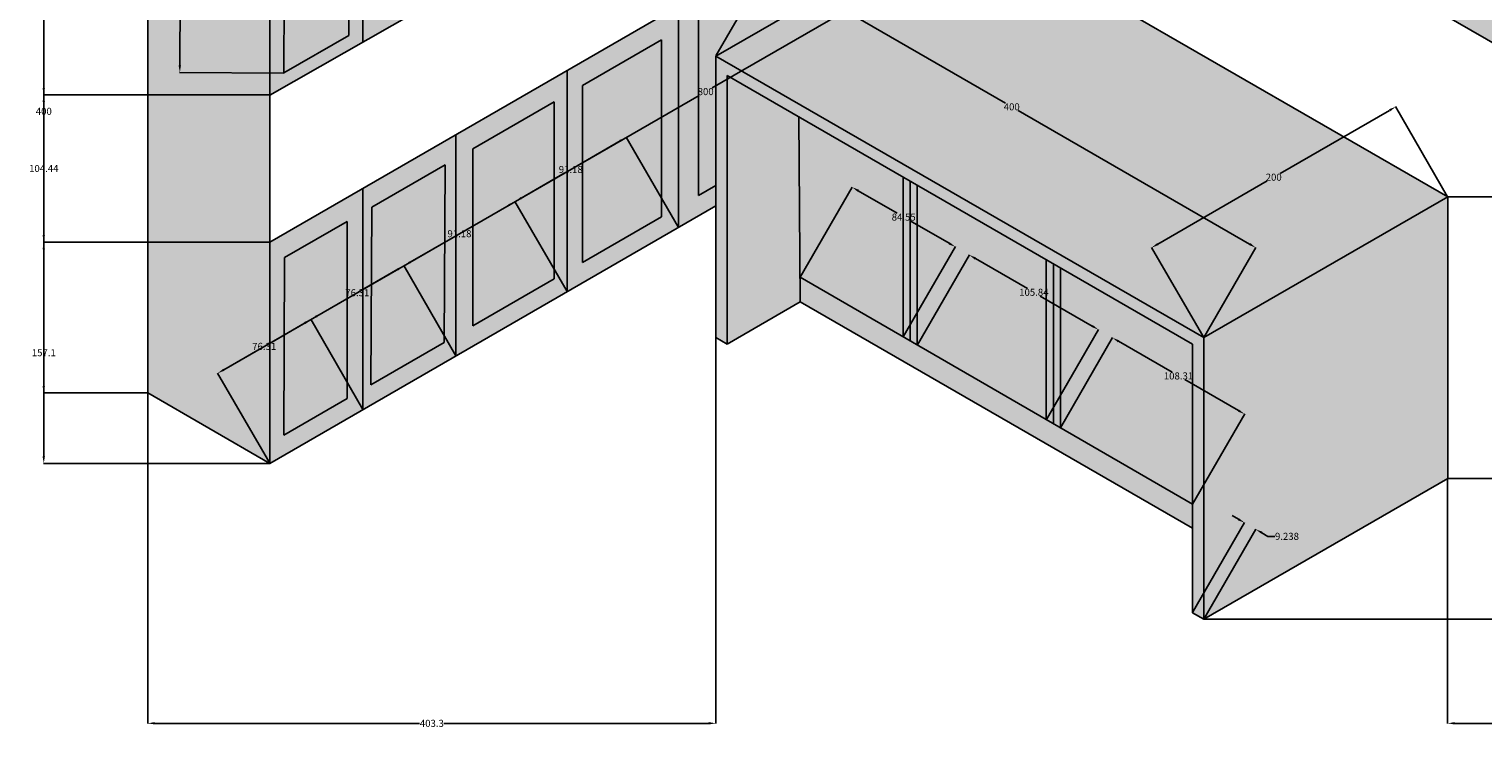
# Model space of a CAD drawing. Units: centimetres. Extents: x -744 to 1642, y 210 to 1375.
# Tile 1 of 8: x -744 to 288, y 210 to 707. Entities that reach past the tile are written whole.
import ezdxf

# ---------------------------------------------------------------- set-up
doc = ezdxf.new("R2010")
doc.units = ezdxf.units.CM
doc.header["$MEASUREMENT"] = 0
for name, color, linetype, lineweight in [('A-ANNO-DIMS', 2, 'Continuous', 18), ('A-EQPM-PATT', 9, 'Continuous', 13), ('A-FURN', 7, 'Continuous', 25), ('A-FURN-PATT', 30, 'Continuous', 13), ('A-WALL-PATT', 61, 'Continuous', 13)]:
    doc.layers.add(name, color=color, linetype=linetype, lineweight=lineweight)
doc.styles.get("Standard").update_dxf_attribs({"font": 'arial.ttf'})
doc.dimstyles.get("Standard").update_dxf_attribs({"dimtxt": 5, "dimasz": 5, "dimexe": 0.18, "dimexo": 0.0625, "dimgap": 0.09, "dimtad": 0, "dimtih": 1, "dimtoh": 1, "dimdec": 0, "dimzin": 0, "dimdsep": 46, "dimtxsty": 'Standard', "dimcen": 0.09, "dimadec": 0, "dimazin": 0, "dimtfac": 1, "dimtdec": 0, "dimtofl": 0, "dimtmove": 0, "dimatfit": 3, "dimfxl": 1, "dimtolj": 1, "dimtzin": 0, "dimarcsym": 0})

# ---------------------------------------------------------------- blocks, each defined once
blk = doc.blocks.new('*D8')
at = {"layer": 'A-ANNO-DIMS', "color": 0, "lineweight": -2, "transparency": 16777216}
for p, q in [((-256.7, 687.4), (-256.7, 213.5)), ((-660, 448.2), (-660, 213.5)), ((-655, 213.6), (-467, 213.6)), ((-261.7, 213.6), (-449.7, 213.6))]:
    blk.add_line(p, q, dxfattribs=at)
at = {"layer": 'A-ANNO-DIMS', "color": 0, "transparency": 16777216}
for points in [[(-655, 214.5), (-655, 212.8), (-660, 213.6)], [(-261.7, 214.5), (-261.7, 212.8), (-256.7, 213.6)]]:
    blk.add_solid(points, dxfattribs=at)
at = {"layer": 'Defpoints', "color": 0, "transparency": 16777216}
for p in [(-256.7, 687.5), (-660, 448.2), (-256.7, 213.6)]:
    blk.add_point(p, dxfattribs=at)
at = {"layer": 'A-ANNO-DIMS', "color": 0, "transparency": 16777216, "insert": (-458.3, 213.6), "char_height": 5, "attachment_point": 5}
blk.add_mtext('\\A1;403.3', dxfattribs=at)
blk = doc.blocks.new('*D9')
at = {"layer": 'A-ANNO-DIMS', "color": 0, "lineweight": -2, "transparency": 16777216}
for p, q in [((812.3, 498.2), (812.3, 213.5)), ((262.9, 387.4), (262.9, 213.5)), ((267.9, 213.6), (529.1, 213.6)), ((807.3, 213.6), (546.1, 213.6))]:
    blk.add_line(p, q, dxfattribs=at)
at = {"layer": 'A-ANNO-DIMS', "color": 0, "transparency": 16777216}
for points in [[(267.9, 214.5), (267.9, 212.8), (262.9, 213.6)], [(807.3, 214.5), (807.3, 212.8), (812.3, 213.6)]]:
    blk.add_solid(points, dxfattribs=at)
at = {"layer": 'Defpoints', "color": 0, "transparency": 16777216}
for p in [(812.3, 498.2), (262.9, 387.5), (812.3, 213.6)]:
    blk.add_point(p, dxfattribs=at)
at = {"layer": 'A-ANNO-DIMS', "color": 0, "transparency": 16777216, "insert": (537.6, 213.6), "char_height": 5, "attachment_point": 5}
blk.add_mtext('\\A1;549.3', dxfattribs=at)
blk = doc.blocks.new('*D10')
at = {"layer": 'A-ANNO-DIMS', "color": 0, "lineweight": -2, "transparency": 16777216}
for p, q in [((119.5, 1298.2), (886.3, 1298.2)), ((886.1, 1293.2), (886.1, 795.5)), ((886.1, 292.5), (886.1, 790.2)), ((89.8, 287.5), (886.3, 287.5))]:
    blk.add_line(p, q, dxfattribs=at)
at = {"layer": 'A-ANNO-DIMS', "color": 0, "transparency": 16777216}
for points in [[(885.3, 1293.2), (886.9, 1293.2), (886.1, 1298.2)], [(885.3, 292.5), (886.9, 292.5), (886.1, 287.5)]]:
    blk.add_solid(points, dxfattribs=at)
at = {"layer": 'Defpoints', "color": 0, "transparency": 16777216}
for p in [(119.4, 1298.2), (886.1, 1298.2), (89.7, 287.5)]:
    blk.add_point(p, dxfattribs=at)
at = {"layer": 'A-ANNO-DIMS', "color": 0, "transparency": 16777216, "insert": (886.1, 792.9), "char_height": 5, "attachment_point": 5}
blk.add_mtext('\\A1;1010.7', dxfattribs=at)
blk = doc.blocks.new('*D11')
at = {"layer": 'A-ANNO-DIMS', "color": 0, "lineweight": -2, "transparency": 16777216}
for p, q in [((-660.1, 848.2), (-734, 848.2)), ((-733.8, 843.2), (-733.8, 650.9)), ((-733.8, 453.2), (-733.8, 645.6)), ((-660.1, 448.2), (-734, 448.2))]:
    blk.add_line(p, q, dxfattribs=at)
at = {"layer": 'A-ANNO-DIMS', "color": 0, "transparency": 16777216}
for points in [[(-734.7, 843.2), (-733, 843.2), (-733.8, 848.2)], [(-734.7, 453.2), (-733, 453.2), (-733.8, 448.2)]]:
    blk.add_solid(points, dxfattribs=at)
at = {"layer": 'Defpoints', "color": 0, "transparency": 16777216}
for p in [(-733.8, 848.2), (-660, 848.2), (-660, 448.2)]:
    blk.add_point(p, dxfattribs=at)
at = {"layer": 'A-ANNO-DIMS', "color": 0, "transparency": 16777216, "insert": (-733.8, 648.2), "char_height": 5, "attachment_point": 5}
blk.add_mtext('\\A1;400', dxfattribs=at)
blk = doc.blocks.new('*D12')
at = {"layer": 'A-ANNO-DIMS', "color": 0, "lineweight": -2, "transparency": 16777216}
for p, q in [((-573.4, 798.2), (-734, 798.2)), ((-733.8, 793.2), (-733.8, 731.7)), ((-733.8, 664.8), (-733.8, 726.4)), ((-573.4, 659.8), (-734, 659.8))]:
    blk.add_line(p, q, dxfattribs=at)
at = {"layer": 'A-ANNO-DIMS', "color": 0, "transparency": 16777216}
for points in [[(-734.7, 793.2), (-733, 793.2), (-733.8, 798.2)], [(-734.7, 664.8), (-733, 664.8), (-733.8, 659.8)]]:
    blk.add_solid(points, dxfattribs=at)
at = {"layer": 'Defpoints', "color": 0, "transparency": 16777216}
for p in [(-573.4, 798.2), (-733.8, 659.8), (-573.4, 659.8)]:
    blk.add_point(p, dxfattribs=at)
at = {"layer": 'A-ANNO-DIMS', "color": 0, "transparency": 16777216, "insert": (-733.8, 729), "char_height": 5, "attachment_point": 5}
blk.add_mtext('\\A1;138.45', dxfattribs=at)
blk = doc.blocks.new('*D13')
at = {"layer": 'A-ANNO-DIMS', "color": 0, "lineweight": -2, "transparency": 16777216}
for p, q in [((-573.4, 659.8), (-734, 659.8)), ((-733.8, 654.8), (-733.8, 610.2)), ((-733.8, 560.3), (-733.8, 604.9)), ((-573.4, 555.3), (-734, 555.3))]:
    blk.add_line(p, q, dxfattribs=at)
at = {"layer": 'A-ANNO-DIMS', "color": 0, "transparency": 16777216}
for points in [[(-734.7, 654.8), (-733, 654.8), (-733.8, 659.8)], [(-734.7, 560.3), (-733, 560.3), (-733.8, 555.3)]]:
    blk.add_solid(points, dxfattribs=at)
at = {"layer": 'Defpoints', "color": 0, "transparency": 16777216}
for p in [(-573.4, 659.8), (-733.8, 555.3), (-573.4, 555.3)]:
    blk.add_point(p, dxfattribs=at)
at = {"layer": 'A-ANNO-DIMS', "color": 0, "transparency": 16777216, "insert": (-733.8, 607.6), "char_height": 5, "attachment_point": 5}
blk.add_mtext('\\A1;104.44', dxfattribs=at)
blk = doc.blocks.new('*D14')
at = {"layer": 'A-ANNO-DIMS', "color": 0, "lineweight": -2, "transparency": 16777216}
for p, q in [((-573.4, 555.3), (-734, 555.3)), ((-733.8, 550.3), (-733.8, 479.4)), ((-733.8, 403.2), (-733.8, 474.1)), ((-573.4, 398.2), (-734, 398.2))]:
    blk.add_line(p, q, dxfattribs=at)
at = {"layer": 'A-ANNO-DIMS', "color": 0, "transparency": 16777216}
for points in [[(-734.7, 550.3), (-733, 550.3), (-733.8, 555.3)], [(-734.7, 403.2), (-733, 403.2), (-733.8, 398.2)]]:
    blk.add_solid(points, dxfattribs=at)
at = {"layer": 'Defpoints', "color": 0, "transparency": 16777216}
for p in [(-573.4, 555.3), (-733.8, 398.2), (-573.4, 398.2)]:
    blk.add_point(p, dxfattribs=at)
at = {"layer": 'A-ANNO-DIMS', "color": 0, "transparency": 16777216, "insert": (-733.8, 476.8), "char_height": 5, "attachment_point": 5}
blk.add_mtext('\\A1;157.1', dxfattribs=at)
blk = doc.blocks.new('*D16')
at = {"layer": 'A-ANNO-DIMS', "color": 0, "lineweight": -2, "transparency": 16777216}
for p, q in [((78.2, 859.7), (-259.3, 664.8)), ((119.4, 798.3), (82.4, 862.3)), ((-606, 464.7), (-268.5, 659.5)), ((-573.4, 398.3), (-610.4, 462.3))]:
    blk.add_line(p, q, dxfattribs=at)
at = {"layer": 'A-ANNO-DIMS', "color": 0, "transparency": 16777216}
for points in [[(77.8, 860.4), (78.6, 859), (82.5, 862.2)], [(-606.4, 465.4), (-605.6, 464), (-610.3, 462.2)]]:
    blk.add_solid(points, dxfattribs=at)
at = {"layer": 'Defpoints', "color": 0, "transparency": 16777216}
for p in [(82.5, 862.2), (119.4, 798.2), (-573.4, 398.2)]:
    blk.add_point(p, dxfattribs=at)
at = {"layer": 'A-ANNO-DIMS', "color": 0, "transparency": 16777216, "insert": (-263.9, 662.2), "char_height": 5, "attachment_point": 5}
blk.add_mtext('\\A1;800', dxfattribs=at)
blk = doc.blocks.new('*D23')
at = {"layer": 'A-ANNO-DIMS', "color": 0, "lineweight": -2, "transparency": 16777216}
for p, q in [((-256.7, 687.5), (-219.7, 751.6)), ((-215.4, 748.9), (-51.1, 654.1)), ((122.3, 553.9), (-42, 648.8)), ((89.8, 487.5), (126.7, 551.6))]:
    blk.add_line(p, q, dxfattribs=at)
at = {"layer": 'A-ANNO-DIMS', "color": 0, "transparency": 16777216}
for points in [[(-215, 749.7), (-215.9, 748.2), (-219.8, 751.4)], [(122.7, 554.7), (121.9, 553.2), (126.6, 551.4)]]:
    blk.add_solid(points, dxfattribs=at)
at = {"layer": 'Defpoints', "color": 0, "transparency": 16777216}
for p in [(-256.7, 687.5), (126.6, 551.4), (89.7, 487.5)]:
    blk.add_point(p, dxfattribs=at)
at = {"layer": 'A-ANNO-DIMS', "color": 0, "transparency": 16777216, "insert": (-46.6, 651.4), "char_height": 5, "attachment_point": 5}
blk.add_mtext('\\A1;400', dxfattribs=at)
blk = doc.blocks.new('*D24')
at = {"layer": 'A-ANNO-DIMS', "color": 0, "lineweight": -2, "transparency": 16777216}
for p, q in [((262.9, 587.5), (225.9, 651.6)), ((221.7, 648.9), (144, 604.1)), ((57.1, 553.9), (134.8, 598.8)), ((89.7, 487.5), (52.7, 551.6))]:
    blk.add_line(p, q, dxfattribs=at)
at = {"layer": 'A-ANNO-DIMS', "color": 0, "transparency": 16777216}
for points in [[(221.3, 649.7), (222.1, 648.2), (226, 651.4)], [(56.7, 554.7), (57.5, 553.2), (52.8, 551.4)]]:
    blk.add_solid(points, dxfattribs=at)
at = {"layer": 'Defpoints', "color": 0, "transparency": 16777216}
for p in [(226, 651.4), (262.9, 587.5), (89.7, 487.5)]:
    blk.add_point(p, dxfattribs=at)
at = {"layer": 'A-ANNO-DIMS', "color": 0, "transparency": 16777216, "insert": (139.4, 601.4), "char_height": 5, "attachment_point": 5}
blk.add_mtext('\\A1;200', dxfattribs=at)
blk = doc.blocks.new('*D25')
at = {"layer": 'A-ANNO-DIMS', "color": 0, "lineweight": -2, "transparency": 16777216}
for p, q in [((263, 587.5), (337, 587.5)), ((336.8, 582.5), (336.8, 490.1)), ((336.8, 392.5), (336.8, 484.8)), ((263, 387.5), (337, 387.5))]:
    blk.add_line(p, q, dxfattribs=at)
at = {"layer": 'A-ANNO-DIMS', "color": 0, "transparency": 16777216}
for points in [[(335.9, 582.5), (337.6, 582.5), (336.8, 587.5)], [(335.9, 392.5), (337.6, 392.5), (336.8, 387.5)]]:
    blk.add_solid(points, dxfattribs=at)
at = {"layer": 'Defpoints', "color": 0, "transparency": 16777216}
for p in [(262.9, 587.5), (262.9, 387.5), (336.8, 387.5)]:
    blk.add_point(p, dxfattribs=at)
at = {"layer": 'A-ANNO-DIMS', "color": 0, "transparency": 16777216, "insert": (336.8, 487.5), "char_height": 5, "attachment_point": 5}
blk.add_mtext('\\A1;200', dxfattribs=at)
blk = doc.blocks.new('*D60')
at = {"layer": 'A-ANNO-DIMS', "color": 0, "lineweight": -2, "transparency": 16777216}
for p, q in [((-548.6, 497.8), (-572.7, 483.9)), ((-507.3, 436.4), (-544.3, 500.5)), ((-606, 464.7), (-581.8, 478.6)), ((-573.4, 398.3), (-610.4, 462.3))]:
    blk.add_line(p, q, dxfattribs=at)
at = {"layer": 'A-ANNO-DIMS', "color": 0, "transparency": 16777216}
for points in [[(-549, 498.6), (-548.1, 497.1), (-544.2, 500.3)], [(-606.4, 465.4), (-605.6, 464), (-610.3, 462.2)]]:
    blk.add_solid(points, dxfattribs=at)
at = {"layer": 'Defpoints', "color": 0, "transparency": 16777216}
for p in [(-544.2, 500.3), (-507.3, 436.4), (-573.4, 398.2)]:
    blk.add_point(p, dxfattribs=at)
at = {"layer": 'A-ANNO-DIMS', "color": 0, "transparency": 16777216, "insert": (-577.3, 481.3), "char_height": 5, "attachment_point": 5}
blk.add_mtext('\\A1;76.31', dxfattribs=at)
blk = doc.blocks.new('*D61')
at = {"layer": 'A-ANNO-DIMS', "color": 0, "lineweight": -2, "transparency": 16777216}
for p, q in [((-441.2, 474.6), (-478.2, 538.7)), ((-482.5, 536), (-506.6, 522.1)), ((-539.9, 502.8), (-515.8, 516.8)), ((-507.3, 436.4), (-544.3, 500.5))]:
    blk.add_line(p, q, dxfattribs=at)
at = {"layer": 'A-ANNO-DIMS', "color": 0, "transparency": 16777216}
for points in [[(-482.9, 536.7), (-482, 535.3), (-478.1, 538.5)], [(-540.3, 503.6), (-539.5, 502.1), (-544.2, 500.3)]]:
    blk.add_solid(points, dxfattribs=at)
at = {"layer": 'Defpoints', "color": 0, "transparency": 16777216}
for p in [(-478.1, 538.5), (-441.2, 474.5), (-507.3, 436.4)]:
    blk.add_point(p, dxfattribs=at)
at = {"layer": 'A-ANNO-DIMS', "color": 0, "transparency": 16777216, "insert": (-511.2, 519.4), "char_height": 5, "attachment_point": 5}
blk.add_mtext('\\A1;76.31', dxfattribs=at)
blk = doc.blocks.new('*D62')
at = {"layer": 'A-ANNO-DIMS', "color": 0, "lineweight": -2, "transparency": 16777216}
for p, q in [((-403.5, 581.6), (-434.1, 563.9)), ((-362.3, 520.2), (-399.3, 584.2)), ((-473.8, 541), (-443.2, 558.7)), ((-441.2, 474.6), (-478.2, 538.7))]:
    blk.add_line(p, q, dxfattribs=at)
at = {"layer": 'A-ANNO-DIMS', "color": 0, "transparency": 16777216}
for points in [[(-403.9, 582.3), (-403.1, 580.9), (-399.2, 584.1)], [(-474.2, 541.7), (-473.4, 540.3), (-478.1, 538.5)]]:
    blk.add_solid(points, dxfattribs=at)
at = {"layer": 'Defpoints', "color": 0, "transparency": 16777216}
for p in [(-399.2, 584.1), (-362.2, 520.1), (-441.2, 474.5)]:
    blk.add_point(p, dxfattribs=at)
at = {"layer": 'A-ANNO-DIMS', "color": 0, "transparency": 16777216, "insert": (-438.7, 561.3), "char_height": 5, "attachment_point": 5}
blk.add_mtext('\\A1;91.18', dxfattribs=at)
blk = doc.blocks.new('*D63')
at = {"layer": 'A-ANNO-DIMS', "color": 0, "lineweight": -2, "transparency": 16777216}
for p, q in [((-283.3, 565.8), (-320.3, 629.8)), ((-324.5, 627.2), (-355.1, 609.5)), ((-394.8, 586.6), (-364.3, 604.2)), ((-362.3, 520.2), (-399.3, 584.2))]:
    blk.add_line(p, q, dxfattribs=at)
at = {"layer": 'A-ANNO-DIMS', "color": 0, "transparency": 16777216}
for points in [[(-325, 627.9), (-324.1, 626.5), (-320.2, 629.7)], [(-395.3, 587.3), (-394.4, 585.9), (-399.2, 584.1)]]:
    blk.add_solid(points, dxfattribs=at)
at = {"layer": 'Defpoints', "color": 0, "transparency": 16777216}
for p in [(-320.2, 629.7), (-283.3, 565.7), (-362.2, 520.1)]:
    blk.add_point(p, dxfattribs=at)
at = {"layer": 'A-ANNO-DIMS', "color": 0, "transparency": 16777216, "insert": (-359.7, 606.9), "char_height": 5, "attachment_point": 5}
blk.add_mtext('\\A1;91.18', dxfattribs=at)
blk = doc.blocks.new('*D65')
at = {"layer": 'A-ANNO-DIMS', "color": 0, "lineweight": -2, "transparency": 16777216}
for p, q in [((-562.9, 787.1), (-636.9, 787.5)), ((-636.7, 782.5), (-637, 734.3)), ((-637.2, 680.8), (-637, 729)), ((-563.5, 675.4), (-637.4, 675.8))]:
    blk.add_line(p, q, dxfattribs=at)
at = {"layer": 'A-ANNO-DIMS', "color": 0, "transparency": 16777216}
for points in [[(-637.6, 782.5), (-635.9, 782.5), (-636.7, 787.5)], [(-638.1, 680.8), (-636.4, 680.8), (-637.2, 675.8)]]:
    blk.add_solid(points, dxfattribs=at)
at = {"layer": 'Defpoints', "color": 0, "transparency": 16777216}
for p in [(-636.7, 787.5), (-562.9, 787.1), (-563.4, 675.4)]:
    blk.add_point(p, dxfattribs=at)
at = {"layer": 'A-ANNO-DIMS', "color": 0, "transparency": 16777216, "insert": (-637, 731.6), "char_height": 5, "attachment_point": 5}
blk.add_mtext('\\A1;111.68', dxfattribs=at)
blk = doc.blocks.new('*D66')
at = {"layer": 'A-ANNO-DIMS', "color": 0, "lineweight": -2, "transparency": 16777216}
for p, q in [((81.8, 292.2), (118.7, 356.2)), ((89.8, 287.5), (126.7, 351.6)), ((114.3, 358.6), (110, 361.1)), ((131, 348.9), (135.3, 346.4)), ((135.3, 346.4), (140.3, 346.4))]:
    blk.add_line(p, q, dxfattribs=at)
at = {"layer": 'A-ANNO-DIMS', "color": 0, "transparency": 16777216}
for points in [[(114.7, 359.3), (113.9, 357.8), (118.6, 356.1)], [(131.4, 349.7), (130.6, 348.2), (126.6, 351.4)]]:
    blk.add_solid(points, dxfattribs=at)
at = {"layer": 'Defpoints', "color": 0, "transparency": 16777216}
for p in [(126.6, 351.4), (81.7, 292.1), (89.7, 287.5)]:
    blk.add_point(p, dxfattribs=at)
at = {"layer": 'A-ANNO-DIMS', "color": 0, "transparency": 16777216, "insert": (148.8, 346.4), "char_height": 5, "attachment_point": 5}
blk.add_mtext('\\A1;9.238', dxfattribs=at)
blk = doc.blocks.new('*D67')
at = {"layer": 'A-ANNO-DIMS', "color": 0, "lineweight": -2, "transparency": 16777216}
for p, q in [((-196.8, 530.4), (-159.8, 594.4)), ((-155.6, 591.8), (-127.9, 575.8)), ((-91, 554.5), (-118.7, 570.5)), ((-123.6, 488.1), (-86.6, 552.1))]:
    blk.add_line(p, q, dxfattribs=at)
at = {"layer": 'A-ANNO-DIMS', "color": 0, "transparency": 16777216}
for points in [[(-155.1, 592.5), (-156, 591.1), (-159.9, 594.3)], [(-90.6, 555.2), (-91.4, 553.7), (-86.7, 552)]]:
    blk.add_solid(points, dxfattribs=at)
at = {"layer": 'Defpoints', "color": 0, "transparency": 16777216}
for p in [(-86.7, 552), (-196.9, 530.3), (-123.7, 488)]:
    blk.add_point(p, dxfattribs=at)
at = {"layer": 'A-ANNO-DIMS', "color": 0, "transparency": 16777216, "insert": (-123.3, 573.1), "char_height": 5, "attachment_point": 5}
blk.add_mtext('\\A1;84.55', dxfattribs=at)
blk = doc.blocks.new('*D68')
at = {"layer": 'A-ANNO-DIMS', "color": 0, "lineweight": -2, "transparency": 16777216}
for p, q in [((-113.6, 482.3), (-76.6, 546.3)), ((-72.4, 543.7), (-35.5, 522.3)), ((10.6, 495.7), (-26.3, 517)), ((-22, 429.3), (15, 493.3))]:
    blk.add_line(p, q, dxfattribs=at)
at = {"layer": 'A-ANNO-DIMS', "color": 0, "transparency": 16777216}
for points in [[(-72, 544.4), (-72.8, 542.9), (-76.7, 546.2)], [(11, 496.4), (10.2, 495), (14.9, 493.2)]]:
    blk.add_solid(points, dxfattribs=at)
at = {"layer": 'Defpoints', "color": 0, "transparency": 16777216}
for p in [(14.9, 493.2), (-113.7, 482.2), (-22, 429.3)]:
    blk.add_point(p, dxfattribs=at)
at = {"layer": 'A-ANNO-DIMS', "color": 0, "transparency": 16777216, "insert": (-30.9, 519.7), "char_height": 5, "attachment_point": 5}
blk.add_mtext('\\A1;105.84', dxfattribs=at)
blk = doc.blocks.new('*D69')
at = {"layer": 'A-ANNO-DIMS', "color": 0, "lineweight": -2, "transparency": 16777216}
for p, q in [((-12, 423.5), (25, 487.6)), ((29.3, 484.9), (67.2, 462.9)), ((114.4, 435.7), (76.4, 457.7)), ((81.8, 369.3), (118.8, 433.3))]:
    blk.add_line(p, q, dxfattribs=at)
at = {"layer": 'A-ANNO-DIMS', "color": 0, "transparency": 16777216}
for points in [[(29.7, 485.6), (28.8, 484.2), (24.9, 487.4)], [(114.8, 436.4), (113.9, 435), (118.7, 433.2)]]:
    blk.add_solid(points, dxfattribs=at)
at = {"layer": 'Defpoints', "color": 0, "transparency": 16777216}
for p in [(-12, 423.5), (118.7, 433.2), (81.7, 369.3)]:
    blk.add_point(p, dxfattribs=at)
at = {"layer": 'A-ANNO-DIMS', "color": 0, "transparency": 16777216, "insert": (71.8, 460.3), "char_height": 5, "attachment_point": 5}
blk.add_mtext('\\A1;108.31', dxfattribs=at)

msp = doc.modelspace()

# ---------------------------------------------------------------- hatches: boundary and pattern name
at = {"layer": 'A-EQPM-PATT'}
h = msp.add_hatch(color=256, dxfattribs=at)
h.dxf.hatch_style = 1
h.paths.add_polyline_path([(3.1189, 737.4813), (-83.4836, 787.4813), (-256.6887, 687.4813), (89.7215, 487.4813), (262.9266, 587.4813)])
h.paths.add_polyline_path([(-197.7282, 644.2029), (-248.6887, 673.6249), (-248.6887, 482.8625), (-196.7272, 512.8625)])
h.paths.add_polyline_path([(262.9266, 587.4813), (89.7215, 487.4813), (89.7215, 287.4813), (262.9266, 387.4813)])
at = {"layer": 'A-FURN-PATT'}
h = msp.add_hatch(color=256, dxfattribs=at)
h.dxf.hatch_style = 1
h.paths.add_polyline_path([(709.906, 763.421), (709.906, 833.5619), (614.425, 888.6879), (614.425, 818.5469)])
h.paths.add_polyline_path([(482.0889, 965.0922), (482.0889, 894.9512), (580.3491, 838.2207), (580.3491, 908.3616)])
h.paths.add_polyline_path([(455.661, 989.3482), (391.7403, 1026.2528), (391.7403, 905.908), (455.661, 869.0034)])
h.paths.add_polyline_path([(367.6025, 1038.9798), (305.4698, 1074.8522), (305.4698, 959.5913), (367.6025, 923.719)])
h.paths.add_polyline_path([(283.2252, 1090.8212), (213.1748, 1130.1519), (213.1748, 1010.3029), (283.2252, 969.8593)])
h.paths.add_polyline_path([(197.085, 1142.1995), (128.5906, 1179.2565), (128.5906, 1060.1567), (197.085, 1020.6114)])
h.paths.add_polyline_path([(111.6616, 1060.697), (111.6616, 1182.612), (67.1993, 1156.9417), (67.1993, 1033.9561)])
h.paths.add_polyline_path([(51.1364, 1025.5999), (51.1364, 1146.3882), (8.133, 1121.5602), (10.63, 1002.2135)])
h.paths.add_polyline_path([(-7.1228, 994.0363), (-7.1228, 1112.7639), (-46.1416, 1090.2363), (-45.0502, 972.1389)])
h.paths.add_polyline_path([(-62.5525, 1080.1953), (-112.7586, 1051.2088), (-111.3243, 975.2962), (-98.1787, 959.5025), (-98.1787, 953.5165), (-110.7754, 946.2438), (-110.5757, 935.6761), (-62.5525, 963.4023)])
h.paths.add_polyline_path([(-131.9167, 1043.3731), (-194.3022, 1007.3548), (-194.3022, 960.6093), (-131.9167, 994.0283)])
h.paths.add_polyline_path([(-210.3768, 1001.0803), (-272.1227, 965.4313), (-272.1227, 916.524), (-210.3442, 952.1919)])
h.paths.add_polyline_path([(-295.3923, 940.164), (-352.6194, 907.1238), (-352.6194, 798.1578), (-299.691, 828.716), (-295.3923, 831.1979)])
h.paths.add_polyline_path([(-373.8641, 892.8311), (-430.554, 860.1012), (-428.9419, 756.8396), (-373.8641, 788.6388)])
h.paths.add_polyline_path([(-449.1461, 850.3626), (-500.1893, 820.8928), (-498.1887, 714.0073), (-449.1461, 742.322)])
h.paths.add_polyline_path([(-517.3336, 813.4139), (-562.861, 787.1286), (-563.3952, 675.4493), (-517.3336, 702.043)])
h.paths.add_polyline_path([(-518.4603, 570.0519), (-562.9383, 544.3726), (-563.4408, 418.3375), (-518.4603, 444.307)])
h.paths.add_polyline_path([(-371.5223, 654.8866), (-429.2034, 621.5845), (-429.2034, 495.8395), (-371.5223, 529.1417)])
h.paths.add_polyline_path([(-448.7547, 610.2965), (-500.7971, 580.2498), (-501.5895, 454.0473), (-449.5067, 484.1173)])
h.paths.add_polyline_path([(-351.4436, 666.4791), (-351.4436, 540.7341), (-295.2328, 573.1874), (-295.2328, 698.9324)])
h.paths.add_polyline_path([(-256.6887, 595.4409), (-256.6887, 687.4813), (-215.6652, 711.1662), (-215.6652, 744.8707), (-268.9239, 714.1219), (-268.9239, 588.3769)])
h.paths.add_polyline_path([(-193.7313, 723.8298), (-132.6965, 759.0682), (-132.6965, 792.7727), (-193.7313, 757.5343)])
h.paths.add_polyline_path([(-114.2, 769.7472), (-83.4836, 787.4813), (-73.2438, 781.5694), (-73.2438, 827.0978), (-114.2, 803.4517)])
h.paths.add_polyline_path([(-53.2271, 770.0128), (-7.0224, 743.3364), (-7.0224, 865.3308), (-53.2271, 838.6544)])
h.paths.add_polyline_path([(8.89, 748.7728), (52.5303, 773.9686), (52.5303, 899.7135), (8.89, 874.5177)])
h.paths.add_polyline_path([(68.067, 782.9387), (108.041, 806.0177), (108.041, 931.7626), (68.067, 908.6836)])
h.paths.add_polyline_path([(130.3442, 802.4419), (196.727, 764.1157), (196.727, 896.2228), (130.3442, 934.5489), (130.3442, 927.6391)])
h.paths.add_polyline_path([(220.7637, 875.3463), (220.7637, 755.5756), (282.3763, 720.0036), (282.3763, 835.7573), (282.3763, 840.4873)])
h.paths.add_polyline_path([(307.3754, 826.3434), (307.3754, 705.693), (368.1078, 670.6291), (368.1078, 790.9456)])
h.paths.add_polyline_path([(389.5829, 779.9795), (389.5829, 656.983), (453.252, 620.2237), (453.252, 747.8082)])
h = msp.add_hatch(color=256, dxfattribs=at)
h.dxf.hatch_style = 1
h.paths.add_polyline_path([(-123.6694, 601.445), (-197.7282, 644.2029), (-196.8604, 530.3463), (-123.6694, 488.0238)])
h.paths.add_polyline_path([(-113.6694, 482.2413), (-22.0425, 429.2584), (-22.0425, 542.7707), (-113.6694, 595.6715)])
h.paths.add_polyline_path([(-12.0425, 536.9972), (-12.0425, 423.4759), (81.7215, 369.2572), (81.7215, 482.8625)])
at = {"layer": 'A-WALL-PATT'}
h = msp.add_hatch(color=256, dxfattribs=at)
h.dxf.hatch_style = 1
h.paths.add_polyline_path([(-226.9766, 998.2308), (119.4335, 1198.2308), (292.6386, 1098.2308), (465.8437, 998.2308), (552.4462, 948.2308), (725.6513, 848.2308), (812.2538, 898.2308), (119.4335, 1298.2308), (-659.9893, 848.2308), (-573.3868, 798.2308)])
h.paths.add_polyline_path([(-573.3868, 798.2308), (-659.9893, 848.2308), (-659.9893, 448.2308), (-573.3868, 398.2308)])
h.paths.add_polyline_path([(-507.2972, 836.3877), (-573.3868, 798.2308), (-573.3868, 659.7809), (-507.2972, 697.4412)])
h.paths.add_polyline_path([(-562.861, 787.1286), (-517.3336, 813.4139), (-517.3336, 702.043), (-563.3952, 675.4493)], flags=16)
h.paths.add_polyline_path([(-441.2075, 735.1015), (-441.2075, 874.5446), (-507.2972, 836.3877), (-507.2972, 697.4412)])
h.paths.add_polyline_path([(-500.1893, 820.8928), (-449.1461, 850.3626), (-449.1461, 742.322), (-498.1887, 714.0073)], flags=16)
h.paths.add_polyline_path([(-362.2449, 780.0973), (-362.2449, 920.1337), (-441.2075, 874.5446), (-441.2075, 735.1015)])
h.paths.add_polyline_path([(-430.554, 860.1012), (-373.8641, 892.8311), (-373.8641, 788.6388), (-428.9419, 756.8396)], flags=16)
h.paths.add_polyline_path([(-283.2822, 825.0931), (-283.2822, 965.7228), (-362.2449, 920.1337), (-362.2449, 780.0973)])
h.paths.add_polyline_path([(-352.6194, 798.1578), (-352.6194, 907.1238), (-295.3923, 940.164), (-295.3923, 831.1979), (-299.691, 828.716)], flags=16)
h.paths.add_polyline_path([(-203.882, 947.929), (-203.5655, 1011.7473), (-226.9766, 998.2308), (-283.2822, 965.7228), (-283.2822, 904.7538)], flags=17)
h.paths.add_polyline_path([(-272.1227, 965.4313), (-210.3768, 1001.0803), (-210.3442, 952.1919), (-272.1227, 916.524)], flags=16)
h.paths.add_polyline_path([(-123.8488, 991.4483), (-123.8488, 1057.7717), (-203.5655, 1011.7473), (-203.882, 947.929)], flags=17)
h.paths.add_polyline_path([(-194.3022, 1007.3548), (-131.9167, 1043.3731), (-131.9167, 994.0283), (-194.3022, 960.6093)], flags=16)
h.paths.add_polyline_path([(-112.7586, 1051.2088), (-62.5525, 1080.1953), (-62.5525, 963.4023), (-110.5757, 935.6761), (-110.7754, 946.2438), (-123.8488, 938.6959), (-123.8488, 915.9442), (-53.7716, 955.8768), (-53.7716, 1098.2308), (-123.8488, 1057.7717), (-123.8488, 991.4483), (-123.8488, 990.3436), (-111.3243, 975.2962)], flags=17)
h.paths.add_polyline_path([(1.2011, 1129.9693), (-53.7716, 1098.2308), (-53.7716, 955.8768), (1.4435, 987.3403)], flags=17)
h.paths.add_polyline_path([(-46.1416, 1090.2363), (-7.1228, 1112.7639), (-7.1228, 994.0363), (-45.0502, 972.1389)], flags=16)
h.paths.add_polyline_path([(60.3173, 1164.1001), (1.2011, 1129.9693), (1.4435, 987.3403), (60.3173, 1020.8888)], flags=17)
h.paths.add_polyline_path([(8.133, 1121.5602), (51.1364, 1146.3882), (51.1364, 1025.5999), (10.63, 1002.2135)], flags=16)
h.paths.add_polyline_path([(119.4335, 1054.5754), (119.4335, 1198.2308), (60.3173, 1164.1001), (60.3173, 1020.8888)], flags=17)
h.paths.add_polyline_path([(67.1993, 1156.9417), (111.6616, 1182.612), (111.6616, 1060.697), (67.1993, 1033.9561)], flags=16)
h.paths.add_polyline_path([(206.0361, 1148.2308), (119.4335, 1198.2308), (119.4335, 1054.5754), (206.0361, 1003.7675)], flags=17)
h.paths.add_polyline_path([(128.5906, 1179.2565), (197.085, 1142.1995), (197.085, 1020.6114), (128.5906, 1060.1567)], flags=16)
h.paths.add_polyline_path([(206.0361, 1148.2308), (206.0361, 1003.7675), (292.6386, 952.9596), (292.6386, 1098.2308)], flags=17)
h.paths.add_polyline_path([(213.1748, 1130.1519), (283.2252, 1090.8212), (283.2252, 969.8593), (213.1748, 1010.3029)], flags=16)
h.paths.add_polyline_path([(292.6386, 1098.2308), (292.6386, 952.9596), (378.4066, 902.6412), (379.2411, 1048.2308)], flags=17)
h.paths.add_polyline_path([(305.4698, 1074.8522), (367.6025, 1038.9798), (367.6025, 923.719), (305.4698, 959.5913)], flags=16)
h.paths.add_polyline_path([(379.2411, 1048.2308), (378.4066, 902.6412), (465.8437, 851.3437), (465.8437, 998.2308)], flags=17)
h.paths.add_polyline_path([(391.7403, 1026.2528), (455.661, 989.3482), (455.661, 869.0034), (391.7403, 905.908)], flags=16)
h.paths.add_polyline_path([(552.4462, 948.2308), (465.8437, 998.2308), (465.8437, 891.6699), (595.7475, 816.0455), (595.7475, 923.2308)], flags=17)
h.paths.add_polyline_path([(482.0889, 965.0922), (580.3491, 908.3616), (580.3491, 838.2207), (482.0889, 894.9512)], flags=16)
h.paths.add_polyline_path([(595.7475, 923.2308), (595.7475, 816.0455), (725.6513, 740.4211), (725.6513, 848.2308)])
h.paths.add_polyline_path([(614.425, 888.6879), (709.906, 833.5619), (709.906, 763.421), (614.425, 818.5469)], flags=16)
h.paths.add_polyline_path([(812.2538, 898.2308), (725.6513, 848.2308), (725.6513, 740.4211), (725.6513, 448.2308), (812.2538, 498.2308)])
h.paths.add_polyline_path([(465.8437, 757.085), (377.8609, 807.4399), (376.9558, 649.5503), (465.8437, 598.2308)])
h.paths.add_polyline_path([(389.5829, 779.9795), (453.252, 747.8082), (453.252, 620.2237), (389.5829, 656.983)], flags=16)
h.paths.add_polyline_path([(377.8609, 807.4399), (292.6386, 856.215), (292.6386, 698.2308), (376.9558, 649.5503)])
h.paths.add_polyline_path([(368.1078, 670.6291), (307.3754, 705.693), (307.3754, 826.3434), (368.1078, 790.9456)], flags=16)
h.paths.add_polyline_path([(292.6386, 856.215), (206.0361, 905.7799), (206.0361, 748.2308), (292.6386, 698.2308)])
h.paths.add_polyline_path([(282.3763, 720.0036), (220.7637, 755.5756), (220.7637, 875.3463), (282.3763, 840.4873), (282.3763, 835.7573)], flags=16)
h.paths.add_polyline_path([(206.0361, 905.7799), (119.4335, 955.3449), (119.4335, 798.2308), (206.0361, 748.2308)])
h.paths.add_polyline_path([(196.727, 764.1157), (130.3442, 802.4419), (130.3442, 927.6391), (130.3442, 934.5489), (196.727, 896.2228)], flags=16)
h.paths.add_polyline_path([(119.4335, 955.3449), (60.5235, 921.3332), (60.5235, 764.2191), (119.4335, 798.2308)])
h.paths.add_polyline_path([(108.041, 806.0177), (68.067, 782.9387), (68.067, 908.6836), (108.041, 931.7626)], flags=16)
h.paths.add_polyline_path([(60.5235, 764.2191), (60.5235, 921.3332), (1.6135, 887.3215), (1.867, 738.2042), (3.1189, 737.4813), (8.6656, 734.279)])
h.paths.add_polyline_path([(8.89, 748.7728), (8.89, 874.5177), (52.5303, 899.7135), (52.5303, 773.9686)], flags=16)
h.paths.add_polyline_path([(1.6135, 887.3215), (-61.1176, 851.1036), (-61.1176, 774.5683), (-53.2271, 770.0128), (-53.2271, 838.6544), (-7.0224, 865.3308), (-7.0224, 743.3364), (1.867, 738.2042)])
h.paths.add_polyline_path([(-61.1176, 851.1036), (-123.8488, 814.8858), (-123.8488, 764.1765), (-114.2, 769.7472), (-114.2, 803.4517), (-73.2438, 827.0978), (-73.2438, 781.5694), (-61.1176, 774.5683)])
h.paths.add_polyline_path([(-132.6965, 792.7727), (-132.6965, 759.0682), (-123.8488, 764.1765), (-123.8488, 814.8858), (-203.5655, 768.8613), (-203.5655, 718.152), (-193.7313, 723.8298), (-193.7313, 757.5343)])
h.paths.add_polyline_path([(-203.5655, 768.8613), (-283.2822, 722.8369), (-283.2822, 565.7228), (-256.6887, 581.0766), (-256.6887, 595.4409), (-268.9239, 588.3769), (-268.9239, 714.1219), (-215.6652, 744.8707), (-215.6652, 711.1662), (-203.5655, 718.152)])
h.paths.add_polyline_path([(-283.2822, 722.8369), (-362.2449, 677.2477), (-362.2449, 520.1337), (-283.2822, 565.7228)])
h.paths.add_polyline_path([(-295.2328, 573.1874), (-351.4436, 540.7341), (-351.4436, 666.4791), (-295.2328, 698.9324)], flags=16)
h.paths.add_polyline_path([(-362.2449, 677.2477), (-441.2075, 631.6586), (-441.2075, 474.5446), (-362.2449, 520.1337)])
h.paths.add_polyline_path([(-371.5223, 529.1417), (-429.2034, 495.8395), (-429.2034, 621.5845), (-371.5223, 654.8866)], flags=16)
h.paths.add_polyline_path([(-441.2075, 631.6586), (-507.2972, 593.5018), (-507.2972, 436.3877), (-441.2075, 474.5446)])
h.paths.add_polyline_path([(-448.7547, 610.2965), (-449.5067, 484.1173), (-501.5895, 454.0473), (-500.7971, 580.2498)], flags=16)
h.paths.add_polyline_path([(-507.2972, 593.5018), (-573.3868, 555.3449), (-573.3868, 398.2308), (-507.2972, 436.3877)])
h.paths.add_polyline_path([(-518.4603, 570.0519), (-518.4603, 444.307), (-563.4408, 418.3375), (-562.9383, 544.3726)], flags=16)
h.paths.add_polyline_path([(-118.6694, 598.5582), (-123.6694, 601.445), (-123.6694, 488.0238), (-118.6694, 485.1326)], flags=17)
h.paths.add_polyline_path([(-113.6694, 595.6715), (-118.6694, 598.5582), (-118.6694, 485.1326), (-113.6694, 482.2413)], flags=17)
h.paths.add_polyline_path([(-12.0425, 536.9972), (-17.0425, 539.8839), (-17.0425, 426.3672), (-12.0425, 423.4759)], flags=17)
h.paths.add_polyline_path([(-17.0425, 539.8839), (-22.0425, 542.7707), (-22.0425, 429.2584), (-17.0425, 426.3672)], flags=17)
h.paths.add_polyline_path([(-256.6887, 687.4813), (-256.6887, 487.4813), (-248.6887, 482.8625), (-248.6887, 673.6249), (81.7215, 482.8625), (81.7215, 292.1001), (89.7215, 287.4813), (89.7215, 487.4813)])
h.paths.add_polyline_path([(-196.8604, 530.3463), (-196.7272, 512.8625), (81.7215, 352.1001), (81.7215, 369.2572)], flags=17)

# ---------------------------------------------------------------- linework, layer by layer
at = {"layer": 'A-FURN'}
for p, q in [((119.4335, 955.3449), (-573.3868, 555.3449)), ((-659.9893, 848.2308), (-659.9893, 448.2308)), ((-507.2972, 836.3877), (-507.2972, 697.4412)), ((-573.3868, 659.7809), (-283.2822, 825.0931)), ((-517.3336, 813.4139), (-517.3336, 702.043)), ((-573.3868, 798.2308), (-573.3868, 398.2308)), ((119.4335, 798.2308), (465.8437, 598.2308)), ((-563.3952, 675.4493), (-562.861, 787.1286)), ((-83.4836, 787.4813), (-256.6887, 687.4813)), ((262.9266, 587.4813), (3.1189, 737.4813)), ((-283.2822, 722.8369), (-283.2822, 565.7228)), ((-268.9239, 714.1219), (-268.9239, 588.3769)), ((-517.3336, 702.043), (-563.3952, 675.4493)), ((-351.4436, 666.4791), (-295.2328, 698.9324)), ((-295.2328, 698.9324), (-295.2328, 573.1874)), ((-256.6887, 687.4813), (89.7215, 487.4813)), ((-256.6887, 687.4813), (-256.6887, 487.4813)), ((-362.2449, 677.2477), (-362.2449, 520.1337)), ((-248.6887, 673.6249), (-248.6887, 482.8625)), ((-248.6887, 673.6249), (81.7215, 482.8625)), ((-351.4436, 666.4791), (-351.4436, 540.7341)), ((-429.2034, 621.5845), (-371.5223, 654.8866)), ((-371.5223, 654.8866), (-371.5223, 529.1417)), ((-196.7272, 512.8625), (-197.7282, 644.2029)), ((-441.2075, 631.6586), (-441.2075, 474.5446)), ((-429.2034, 621.5845), (-429.2034, 495.8395)), ((-500.7971, 580.2498), (-448.7547, 610.2965)), ((-448.7547, 610.2965), (-449.5067, 484.1173)), ((-123.6694, 601.445), (-123.6694, 488.0238)), ((-507.2972, 593.5018), (-507.2972, 436.3877)), ((-268.9239, 588.3769), (-256.6887, 595.4409)), ((-118.6694, 598.5582), (-118.6694, 485.1326)), ((-113.6694, 595.6715), (-113.6694, 482.2413)), ((-256.6887, 581.0766), (-573.3868, 398.2308)), ((-500.7971, 580.2498), (-501.5895, 454.0473)), ((89.7215, 487.4813), (262.9266, 587.4813)), ((262.9266, 587.4813), (262.9266, 387.4813)), ((-562.9383, 544.3726), (-518.4603, 570.0519)), ((-518.4603, 570.0519), (-518.4603, 444.307)), ((-351.4436, 540.7341), (-295.2328, 573.1874)), ((-562.9383, 544.3726), (-563.4408, 418.3375)), ((-22.0425, 542.7707), (-22.0425, 429.2584)), ((-17.0425, 539.8839), (-17.0425, 426.3672)), ((-12.0425, 536.9972), (-12.0425, 423.4759)), ((-429.2034, 495.8395), (-371.5223, 529.1417)), ((-196.8604, 530.3463), (81.7215, 369.2572)), ((-248.6887, 482.8625), (-196.7272, 512.8625)), ((-196.7272, 512.8625), (81.7215, 352.1001)), ((-248.6887, 482.8625), (-256.6887, 487.4813)), ((89.7215, 287.4813), (89.7215, 487.4813)), ((-501.5895, 454.0473), (-449.5067, 484.1173)), ((81.7215, 292.1001), (81.7215, 482.8625)), ((-573.3868, 398.2308), (-659.9893, 448.2308)), ((-563.4408, 418.3375), (-518.4603, 444.307)), ((262.9266, 387.4813), (89.7215, 287.4813)), ((89.7215, 287.4813), (81.7215, 292.1001))]:
    msp.add_line(p, q, dxfattribs=at)

# ---------------------------------------------------------------- dimensions: what is measured, and where the dimension line sits
at = {"layer": 'A-ANNO-DIMS'}
for base, p1, p2, angle, override, picture, middle in [((886.1038, 1298.2308), (89.7215, 287.4813), (119.4335, 1298.2308), 90, {"dimdec": 1, "dimlfac": 1, "dimrnd": 0, "dimzin": 0, "dimdsep": 46, "dimlunit": 2}, '*D10', (886.1038, 792.8561)), ((82.5085, 862.1868), (-573.3868, 398.2308), (119.4335, 798.2308), 30, {"dimdec": 0, "dimlfac": 1, "dimrnd": 0, "dimzin": 0, "dimdsep": 46, "dimlunit": 2}, '*D16', (-263.9016, 662.1868)), ((-733.8393, 848.2308), (-659.9893, 448.2308), (-659.9893, 848.2308), 90, {"dimdec": 0, "dimlfac": 1, "dimrnd": 0, "dimzin": 0, "dimdsep": 46, "dimlunit": 2}, '*D11', (-733.8393, 648.2308)), ((-733.8393, 659.7809), (-573.3868, 798.2308), (-573.3868, 659.7809), 90, {"dimdec": 2, "dimlfac": 1, "dimrnd": 0, "dimzin": 0, "dimdsep": 46, "dimlunit": 2}, '*D12', (-733.8393, 729.0058)), ((-636.7102, 787.4819), (-563.3952, 675.4493), (-562.861, 787.1286), 89.725961, {"dimdec": 2, "dimlfac": 1, "dimrnd": 0, "dimzin": 0, "dimdsep": 46, "dimlunit": 2}, '*D65', (-636.9772, 731.6422)), ((126.6465, 551.4373), (-256.6887, 687.4813), (89.7215, 487.4813), 330, {"dimdec": 0, "dimlfac": 1, "dimrnd": 0, "dimzin": 0, "dimdsep": 46, "dimlunit": 2}, '*D23', (-46.5586, 651.4373)), ((-733.8393, 555.3449), (-573.3868, 659.7809), (-573.3868, 555.3449), 90, {"dimdec": 2, "dimlfac": 1, "dimrnd": 0, "dimzin": 0, "dimdsep": 46, "dimlunit": 2}, '*D13', (-733.8393, 607.5629)), ((226.0016, 651.4373), (89.7215, 487.4813), (262.9266, 587.4813), 30, {"dimdec": 0, "dimlfac": 1, "dimrnd": 0, "dimzin": 0, "dimdsep": 46, "dimlunit": 2}, '*D24', (139.399, 601.4373)), ((-320.2072, 629.6788), (-362.2449, 520.1337), (-283.2822, 565.7228), 30, {"dimdec": 2, "dimlfac": 1, "dimrnd": 0, "dimzin": 0, "dimdsep": 46, "dimlunit": 2}, '*D63', (-359.6885, 606.8842)), ((-86.7014, 551.955), (-196.8604, 530.3463), (-123.6694, 488.0238), 329.961495, {"dimdec": 2, "dimlfac": 1, "dimrnd": 0, "dimzin": 0, "dimdsep": 46, "dimlunit": 2}, '*D67', (-123.2969, 573.1162)), ((-399.1699, 584.0897), (-441.2075, 474.5446), (-362.2449, 520.1337), 30, {"dimdec": 2, "dimlfac": 1, "dimrnd": 0, "dimzin": 0, "dimdsep": 46, "dimlunit": 2}, '*D62', (-438.6512, 561.2951)), ((336.7766, 387.4813), (262.9266, 587.4813), (262.9266, 387.4813), 270, {"dimdec": 0, "dimlfac": 1, "dimrnd": 0, "dimzin": 0, "dimdsep": 46, "dimlunit": 2}, '*D25', (336.7766, 487.4813)), ((-733.8393, 398.2308), (-573.3868, 555.3449), (-573.3868, 398.2308), 90, {"dimdec": 1, "dimlfac": 1, "dimrnd": 0, "dimzin": 0, "dimdsep": 46, "dimlunit": 2}, '*D14', (-733.8393, 476.7879)), ((-478.1325, 538.5005), (-507.2972, 436.3877), (-441.2075, 474.5446), 30, {"dimdec": 2, "dimlfac": 1, "dimrnd": 0, "dimzin": 0, "dimdsep": 46, "dimlunit": 2}, '*D61', (-511.1773, 519.4221)), ((14.9255, 493.1895), (-113.6694, 482.2413), (-22.0425, 429.2584), 329.961495, {"dimdec": 2, "dimlfac": 1, "dimrnd": 0, "dimzin": 0, "dimdsep": 46, "dimlunit": 2}, '*D68', (-30.8879, 519.681)), ((-544.2222, 500.3437), (-573.3868, 398.2308), (-507.2972, 436.3877), 30, {"dimdec": 2, "dimlfac": 1, "dimrnd": 0, "dimzin": 0, "dimdsep": 46, "dimlunit": 2}, '*D60', (-577.267, 481.2652)), ((118.6895, 433.1884), (-12.0425, 423.4759), (81.7215, 369.2572), 329.961495, {"dimdec": 2, "dimlfac": 1, "dimrnd": 0, "dimzin": 0, "dimdsep": 46, "dimlunit": 2}, '*D69', (71.8075, 460.2977)), ((126.6465, 351.4373), (81.7215, 292.1001), (89.7215, 287.4813), 330, {"dimdec": 3, "dimlfac": 1, "dimrnd": 0, "dimzin": 0, "dimdsep": 46, "dimlunit": 2}, '*D66', (148.8381, 346.4373))]:
    dim = msp.add_linear_dim(base=base, p1=p1, p2=p2, angle=angle, dimstyle='Standard', override=override, dxfattribs=at)
    dim.commit()
    dim.dimension.update_dxf_attribs({"geometry": picture, "text_midpoint": middle})
for base, p1, p2, picture, middle in [((-256.6887, 213.6313), (-659.9893, 448.2308), (-256.6887, 687.4813), '*D8', (-458.339, 213.6313)), ((812.2538, 213.6313), (262.9266, 387.4813), (812.2538, 498.2308), '*D9', (537.5902, 213.6313))]:
    dim = msp.add_linear_dim(base=base, p1=p1, p2=p2, dimstyle='Standard', override={"dimdec": 1, "dimlfac": 1, "dimrnd": 0, "dimzin": 0, "dimdsep": 46, "dimlunit": 2}, dxfattribs=at)
    dim.commit()
    dim.dimension.update_dxf_attribs({"geometry": picture, "text_midpoint": middle})

doc.saveas('drawing.dxf')
